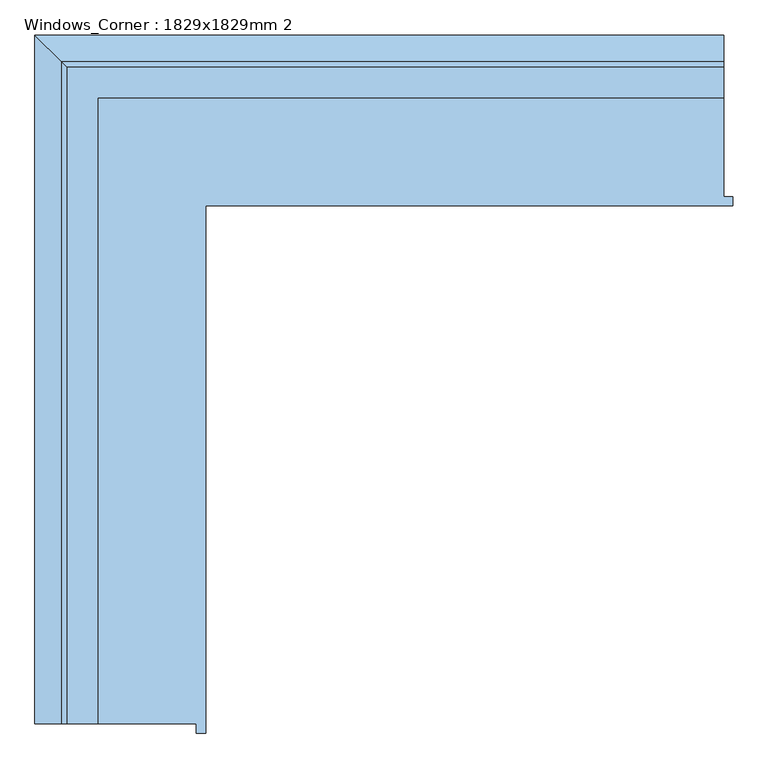
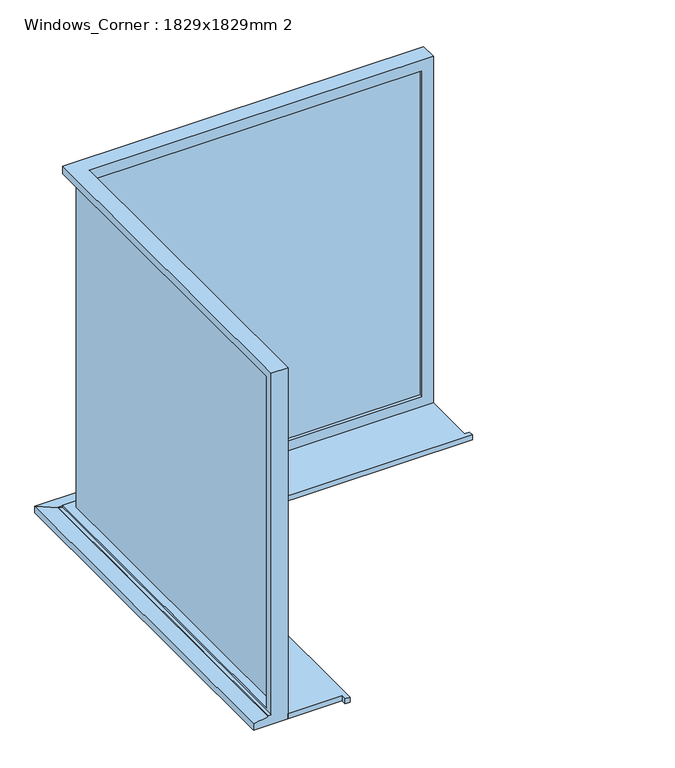
"""IFC4 building model written with IfcOpenShell, lengths in millimetres: window geometry, Windows_Corner : 1829x1829mm 2."""

from ifc_helpers import new_model, si_unit, frame, origin, place, context, project, spatial, polyline, outline, extrude, faceted_brep, source, transform, mapped, element, save


def windows_corner_1829x1829mm_2_98ac2af9(model_context):
    return source(origin(), model_context, "Body", "SolidModel", [
        faceted_brep([(914.4, -108.2044029, 2110.0), (914.4, -25.2044029, 2110.0), (-864.4, -25.2044029, 2110.0), (-864.4, -1804.0044029, 2110.0), (-781.4, -1804.0044029, 2110.0), (-781.4, -108.2044029, 2110.0), (914.4, -25.2044029, 332.2), (-864.4, -25.2044029, 332.2), (-864.4, -25.2044029, 344.2), (874.4, -25.2044029, 344.2), (874.4, -25.2044029, 2070.0), (-864.4, -25.2044029, 2070.0), (874.4, -90.2044029, 2070.0), (-799.4, -90.2044029, 2070.0), (-799.4, -1764.0044029, 2070.0), (-864.4, -1764.0044029, 2070.0), (874.4, -90.2044029, 344.2), (-799.4, -90.2044029, 344.2), (-799.4, -90.2044029, 356.2), (859.4, -90.2044029, 356.2), (859.4, -90.2044029, 2055.0), (-799.4, -90.2044029, 2055.0), (859.4, -108.2044029, 2055.0), (-781.4, -108.2044029, 2055.0), (-781.4, -1749.0044029, 2055.0), (-799.4, -1749.0044029, 2055.0), (859.4, -108.2044029, 356.2), (-781.4, -108.2044029, 356.2), (-781.4, -108.2044029, 281.2), (914.4, -108.2044029, 281.2), (914.4, 62.2955971, 281.2), (914.4, 62.2955971, 315.0088847), (914.4, -10.2044029, 325.9449676), (914.4, -10.2044029, 330.88767), (-781.4, -1804.0044029, 281.2), (-951.9, -1804.0044029, 281.2), (-951.9, 62.2955971, 281.2), (-951.9, 62.2955971, 315.0088847), (-879.4, -10.2044029, 325.9449676), (-879.4, -10.2044029, 330.88767), (-864.4, -1764.0044029, 344.2), (-799.4, -1764.0044029, 344.2), (-799.4, -1749.0044029, 356.2), (-781.4, -1749.0044029, 356.2), (-864.4, -1804.0044029, 332.2), (-879.4, -1804.0044029, 330.88767), (-879.4, -1804.0044029, 325.9449676), (-951.9, -1804.0044029, 315.0088847)], [[[0, 1, 2, 3, 4, 5]], [[6, 7, 8, 9, 10, 11, 2, 1]], [[10, 12, 13, 14, 15, 11]], [[13, 12, 16, 17, 18, 19, 20, 21]], [[20, 22, 23, 24, 25, 21]], [[0, 5, 23, 22, 26, 27, 28, 29]], [[6, 1, 0, 29, 30, 31, 32, 33]], [[10, 9, 16, 12]], [[22, 20, 19, 26]], [[30, 29, 28, 34, 35, 36]], [[31, 30, 36, 37]], [[32, 31, 37, 38]], [[33, 32, 38, 39]], [[6, 33, 39, 7]], [[8, 40, 41, 17, 16, 9]], [[18, 42, 43, 27, 26, 19]], [[35, 34, 4, 3, 44, 45, 46, 47]], [[28, 27, 43, 24, 23, 5, 4, 34]], [[36, 35, 47, 37]], [[38, 37, 47, 46]], [[39, 38, 46, 45]], [[7, 39, 45, 44]], [[8, 7, 44, 3, 2, 11, 15, 40]], [[18, 17, 41, 14, 13, 21, 25, 42]], [[25, 24, 43, 42]], [[15, 14, 41, 40]]]),
        extrude(outline(polyline([(874.4, -90.2044029), (-799.4, -90.2044029), (-799.4, -1764.0044029), (-823.4, -1764.0044029), (-823.4, -66.2044029), (874.4, -66.2044029), (874.4, -90.2044029)])), frame((0.0, 0.0, 344.2), z_axis=(0.0, 0.0, 1.0), x_axis=(1.0, 0.0, 0.0)), (0.0, 0.0, 1.0), 1710.8),
        extrude(outline(polyline([(-781.4, -108.2044029), (914.4, -108.2044029), (914.4, -375.2044029), (939.4, -375.2044029), (939.4, -400.2044029), (-489.4, -400.2044029), (-489.4, -1829.0044029), (-514.4, -1829.0044029), (-514.4, -1804.0044029), (-781.4, -1804.0044029), (-781.4, -108.2044029)])), frame((0.0, 0.0, 281.2), z_axis=(0.0, 0.0, 1.0), x_axis=(1.0, 0.0, 0.0)), (0.0, 0.0, 1.0), 25.0),
    ])


if __name__ == "__main__":
    model = new_model("IFC4")
    model_context = context("Model", 3, world=origin())
    ifc_project = project(units=[si_unit("LENGTHUNIT", "METRE", prefix="MILLI")], contexts=[model_context])
    site = spatial("IfcSite", under=ifc_project)
    building = spatial("IfcBuilding", under=site)
    placement = place(None, origin())
    windows_corner_1829x1829mm_2_shape = windows_corner_1829x1829mm_2_98ac2af9(model_context)
    element("IfcWindow", 1, ObjectType="Windows_Corner : 1829x1829mm 2", at=placement, inside=building, context=model_context, shape_type="MappedRepresentation", body=[
        mapped(windows_corner_1829x1829mm_2_shape, transform((0.0, 0.0, 0.0), x_axis=(1.0, 0.0, 0.0), y_axis=(0.0, 1.0, 0.0), z_axis=(0.0, 0.0, 1.0))),
    ])
    save(model, "model.ifc")

# Revit data of these elements
# Type "Windows_Corner : 1829x1829mm 2"
#   Type Mark = "56"
#   Operation = "UserDefined"
#   Construction Type Id = "GSP4R"
#   Keynote = "L10"
#   Analytic Construction = "1/8 in Pilkington single glazing"
#   Wrap Layers (Ext) from Ext = 0' - 4.03543"
#   Wrap Layers (Int) from Ext = 0' - 6.98819"
#   Window Board Projection = 0' - 0.98425"
#   Window Board Extension = 0' - 0.98425"
#   Wall/Void Thickness [instance default] = 1' - 3.74803"
#   Visual Light Transmittance = 0.9
#   Solar Heat Gain Coefficient = 0.78
#   Rough Width = 6' - 0"
#   Rough Height = 6' - 0"
#   Height = 6' - 0"
#   Width = 6' - 0"
#   Heat Transfer Coefficient (U) = 3.6886 W/(m²·K)
#   Glazing Thickness = 0' - 0.94488"
#   FrameOffset - External = 0' - 1.9685"
#   Frame Depth = 0' - 2.55906"
#   Default Head Height = 6' - 11.07087"
#   Cill Depth = 0' - 3.44488"
#   Define Thermal Properties by = 1
#   Wall Closure = 1
#   Material Trim = Window Frame
#   Material Glass = Glass
#   Material Frame = Window Frame
#   Manufacturer = ""
# Element 1 (IfcWindow, "Windows_Corner : 1829x1829mm 2")
#   Materials on its faces: "Window Frame", "Glass"
# Materials
#   "Window Frame": colour RGB 249 249 249, transparency 0, Keynote = "L10", Cost = 0
#   "Glass": class "Glass", colour RGB 0 128 192, transparency 0.9, Description = "Soda Lime Glass", Cost = 0
